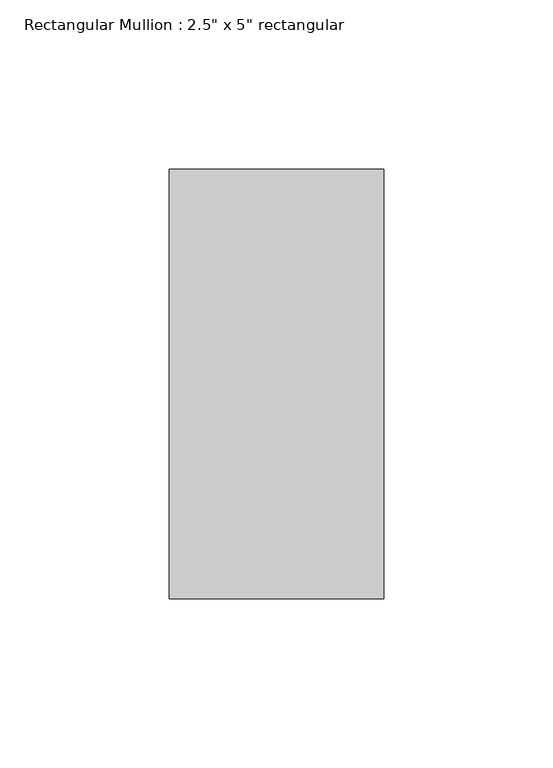
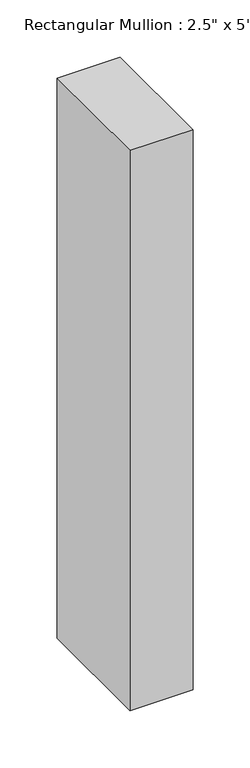
"""IFC4 building model written with IfcOpenShell, lengths in millimetres: member geometry."""

from ifc_helpers import new_model, si_unit, frame, origin, place, context, project, spatial, polyline, outline, extrude, source, transform, mapped, element, save


def member_a400357f(model_context):
    return source(origin(), model_context, "Body", "SweptSolid", [
        extrude(outline(polyline([(0.0, 63.5), (0.0, -63.5), (-63.5, -63.5), (-63.5, 63.5), (0.0, 63.5)])), frame((0.0, 0.0, -596.9), z_axis=(0.0, 0.0, 1.0), x_axis=(1.0, 0.0, 0.0)), (0.0, 0.0, 1.0), 596.9),
    ])


if __name__ == "__main__":
    model = new_model("IFC4")
    model_context = context("Model", 3, world=origin())
    ifc_project = project(units=[si_unit("LENGTHUNIT", "METRE", prefix="MILLI")], contexts=[model_context])
    site = spatial("IfcSite", under=ifc_project)
    building = spatial("IfcBuilding", under=site)
    placement = place(None, origin())
    member_shape = member_a400357f(model_context)
    element("IfcMember", 1, ObjectType="Rectangular Mullion : 2.5\" x 5\" rectangular", at=placement, inside=building, context=model_context, shape_type="MappedRepresentation", body=[
        mapped(member_shape, transform((0.0, 0.0, 0.0), x_axis=(1.0, 0.0, 0.0), y_axis=(0.0, 1.0, 0.0), z_axis=(0.0, 0.0, 1.0))),
    ])
    save(model, "model.ifc")

# Revit data of these elements
# Type "Rectangular Mullion : 2.5\" x 5\" rectangular"
#   built-in parameter 1007304 = 0.416667 (stored number, unit not read)
#   built-in parameter 1007301 = 0.104167 (stored number, unit not read)
#   built-in parameter 1007300 = 0.104167 (stored number, unit not read)
